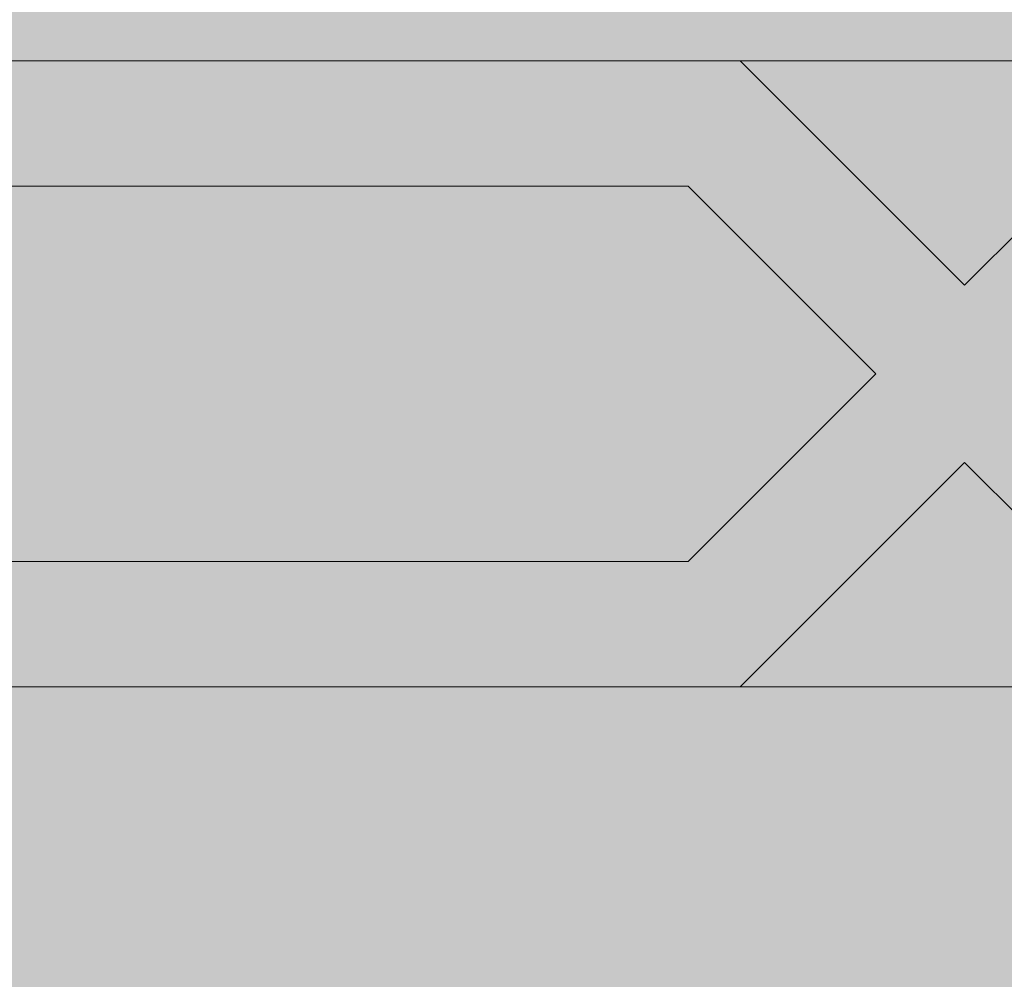
# Model space of a CAD drawing. Units: inches. Extents: x 844 to 2234, y 346 to 1084.
# Tile 81 of 93: x 2001.933 to 2003.94, y 710.971 to 712.926. Entities that reach past the tile are written whole.
import ezdxf

# ---------------------------------------------------------------- set-up
doc = ezdxf.new("R2010")
doc.units = ezdxf.units.IN
doc.header["$MEASUREMENT"] = 0
for name, color, linetype, lineweight in [('A-ANNO-DIMS', 2, 'Continuous', 18), ('furniture', 8, 'Continuous', 18), ('RA-AP-01$0$INT', 35, 'Continuous', 5)]:
    doc.layers.add(name, color=color, linetype=linetype, lineweight=lineweight)
doc.layers.add('RA-AP-01$0$FURN', color=3, linetype='Continuous')
doc.styles.get("Standard").update_dxf_attribs({"font": 'arial.ttf'})
doc.dimstyles.get("Standard").update_dxf_attribs({"dimtxt": 6, "dimasz": 3, "dimexe": 0.18, "dimexo": 0.0625, "dimgap": 0.09, "dimtad": 0, "dimtih": 1, "dimtoh": 1, "dimdec": 1, "dimzin": 0, "dimdsep": 46, "dimlunit": 3, "dimtxsty": 'Standard', "dimblk": 'ARCHTICK', "dimcen": 0.09, "dimadec": 0, "dimazin": 0, "dimtfac": 1, "dimtdec": 1, "dimtofl": 0, "dimtmove": 0, "dimatfit": 3, "dimfxl": 1, "dimtolj": 1, "dimtzin": 0, "dimarcsym": 0})

# ---------------------------------------------------------------- blocks, each defined once
blk = doc.blocks.new('A$C18D01794')
at = {"layer": 'RA-AP-01$0$INT'}
h = blk.add_hatch(color=256, dxfattribs=at)
h.paths.add_polyline_path([(4.355206456958071, -6.156712009588037), (4.355206456958071, -8.056712009588038), (5.455206456958072, -8.056712009588038), (5.455206456958072, -6.156712009588037)])
h.paths.add_polyline_path([(4.405206456958072, -8.006712009588039), (4.405206456958072, -6.206712009588038), (5.405206456958072, -6.206712009588038), (5.405206456958072, -8.006712009588039)], flags=16)
h = blk.add_hatch(color=256, dxfattribs=at)
h.paths.add_polyline_path([(4.505206456958071, -7.585498806127123), (4.46934859260189, -7.549640941759413), (4.505206456958071, -7.513783077414768), (4.505206456958071, -7.381963272220687), (4.469348592616735, -7.346105407867824), (4.505206456958071, -7.310247543514964), (4.505206456958071, -7.178427738324996), (4.469348592586679, -7.142569873965138), (4.505206456952245, -7.106712009588038), (4.476922185709333, -7.106712009588038), (4.455206456960671, -7.128427738343681), (4.433490728198047, -7.106712009588038), (4.405206456946033, -7.106712009588036), (4.441064321339216, -7.142569873969684), (4.40520645695807, -7.178427738362358), (4.405206456958072, -7.310247543472698), (4.441064321364728, -7.346105407867826), (4.40520645695807, -7.381963272262947), (4.40520645695807, -7.513783077378263), (4.441064321354429, -7.549640941786153), (4.405206456958072, -7.585498806170974), (4.405206456958072, -7.717318611286652), (4.441064321333084, -7.753176475673194), (4.405206456958072, -7.789034340036673), (4.405206456958072, -8.006712009588039), (4.644348592588106, -8.006712009588039), (4.680206456964639, -7.970854145211967), (4.716064321341165, -8.006712009588039), (4.869348592586113, -8.006712009588039), (4.905206456964143, -7.970854145210465), (4.941064321342174, -8.006712009588039), (5.094348592587118, -8.006712009588037), (5.130206456963649, -7.970854145211967), (5.166064321340178, -8.006712009588039), (5.405206456958072, -8.006712009588039), (5.405206456958072, -7.789034340024526), (5.369348592595202, -7.753176475673196), (5.40520645695807, -7.717318611298797), (5.40520645695807, -7.585498806158829), (5.369348592573859, -7.549640941786151), (5.40520645695807, -7.51378307739041), (5.40520645695807, -7.381963272250803), (5.36934859256356, -7.346105407867824), (5.405206456958072, -7.310247543484846), (5.405206456958072, -7.178427738350217), (5.369348592589068, -7.142569873969682), (5.405206456982249, -7.106712009588038), (5.376922185730244, -7.106712009588038), (5.355206456967613, -7.128427738343679), (5.333490728218955, -7.10671200958804), (5.305206456976043, -7.106712009588042), (5.341064321341609, -7.142569873965136), (5.305206456958072, -7.178427738337141), (5.305206456958072, -7.310247543502816), (5.34106432131155, -7.346105407867824), (5.305206456958072, -7.381963272232832), (5.30520645695807, -7.513783077402624), (5.341064321326395, -7.549640941759413), (5.305206456958072, -7.585498806139263), (5.305206456958072, -7.717318611299605), (5.341064321347738, -7.753176475677737), (5.305206456958072, -7.78903434007894), (5.30520645695807, -7.906712009588039), (5.166064321336834, -7.906712009588039), (5.130206456963647, -7.942569873961684), (5.094348592590464, -7.906712009588039), (4.941064321338827, -7.906712009588041), (4.905206456964145, -7.942569873963183), (4.869348592589459, -7.906712009588039), (4.716064321337822, -7.906712009588041), (4.680206456964641, -7.942569873961684), (4.644348592591453, -7.906712009588039), (4.505206456958071, -7.906712009588039), (4.505206456958071, -7.789034340066795), (4.469348592580545, -7.753176475677738), (4.505206456958071, -7.717318611311748)])
h.paths.add_polyline_path([(4.485206456974132, -7.709034340046354), (4.45520645695909, -7.739034340051736), (4.425206456974128, -7.709034340057131), (4.425206456993394, -7.593783077384998), (4.45520645699153, -7.563783077396511), (4.485206456993396, -7.593783077408017)], flags=16)
h.paths.add_polyline_path([(4.455206456954537, -7.767318611299197), (4.485206456958242, -7.797318611312542), (4.48520645695951, -7.912569873958716), (4.45520645695415, -7.942569873954422), (4.425206456957888, -7.912569873967813), (4.425206456957888, -7.797318611286197)], flags=16)
h.paths.add_polyline_path([(4.455206456964794, -7.535498806149051), (4.42520645696469, -7.5054988061393), (4.425206456983954, -7.390247543486406), (4.455206456990734, -7.360247543489279), (4.485206456983953, -7.39024754349214), (4.485206456964687, -7.505498806158811)], flags=16)
h.paths.add_polyline_path([(4.499348592588947, -7.926712009585049), (4.636064321340932, -7.926712009585049), (4.666064321342317, -7.956712009586821), (4.636064321343707, -7.986712009585048), (4.499348592575121, -7.986712009585048), (4.469348592591685, -7.956712009591957)], flags=16)
h.paths.add_polyline_path([(4.425206456957888, -7.940854145195974), (4.471064321332215, -7.986712009585049), (4.425206456957888, -7.986712009585049)], flags=16)
h.paths.add_polyline_path([(4.455206456990734, -7.331963272246367), (4.425206456989053, -7.301963272254337), (4.425206456969784, -7.186712009596224), (4.455206456965226, -7.156712009591144), (4.485206456969787, -7.186712009586051), (4.485206456989053, -7.301963272238404)], flags=16)
h.paths.add_polyline_path([(4.72434859258714, -7.926712009586255), (4.861064321340141, -7.926712009586248), (4.891064321340324, -7.956712009586823), (4.861064321340513, -7.986712009586252), (4.724348592586768, -7.986712009586252), (4.694348592586956, -7.956712009586821)], flags=16)
h.paths.add_polyline_path([(4.919348592587961, -7.956712009586821), (4.949348592588145, -7.92671200958625), (5.08606432134115, -7.926712009586253), (5.116064321341327, -7.956712009586823), (5.086064321341519, -7.986712009586252), (4.949348592587774, -7.986712009586252)], flags=16)
h.paths.add_polyline_path([(5.144348592585967, -7.956712009586823), (5.174348592587358, -7.926712009585049), (5.311064321339338, -7.926712009585049), (5.3410643213366, -7.956712009591957), (5.311064321353163, -7.986712009585048), (5.174348592584576, -7.986712009585048)], flags=16)
h.paths.add_polyline_path([(5.32520645693489, -7.593783077408021), (5.355206456936755, -7.563783077396511), (5.385206456934894, -7.593783077384998), (5.38520645695416, -7.709034340057128), (5.355206456969194, -7.739034340051736), (5.325206456954153, -7.709034340046352)], flags=16)
h.paths.add_polyline_path([(5.325206456970042, -7.797318611312542), (5.355206456973747, -7.767318611299197), (5.385206456970398, -7.7973186112862), (5.385206456970398, -7.912569873967816), (5.355206456974136, -7.942569873954422), (5.325206456968778, -7.912569873958716)], flags=16)
h.paths.add_polyline_path([(5.325206456963599, -7.505498806158811), (5.325206456944333, -7.39024754349214), (5.355206456937552, -7.360247543489279), (5.385206456944332, -7.39024754348641), (5.385206456963596, -7.505498806139303), (5.355206456963492, -7.53549880614905)], flags=16)
h.paths.add_polyline_path([(5.32520645693923, -7.301963272238403), (5.3252064569585, -7.186712009586051), (5.355206456963062, -7.156712009591142), (5.3852064569585, -7.186712009596224), (5.385206456939234, -7.301963272254338), (5.355206456937552, -7.331963272246369)], flags=16)
h.paths.add_polyline_path([(5.339348592596071, -7.986712009585048), (5.385206456970398, -7.940854145195972), (5.385206456970396, -7.986712009585048)], flags=16)
h = blk.add_hatch(color=256, dxfattribs=at)
h.paths.add_polyline_path([(4.469348592586677, -7.142569873965136), (4.505206456958073, -7.178427738324996), (4.505206456958071, -7.106712009582215)])
h.paths.add_polyline_path([(4.455206456960671, -7.128427738343681), (4.476922185709333, -7.106712009588038), (4.433490728198045, -7.106712009588038)])
h.paths.add_polyline_path([(4.405206456958073, -7.178427738362358), (4.441064321339218, -7.142569873969684), (4.40520645695807, -7.106712009600073)])
h.paths.add_polyline_path([(4.425206456989053, -7.301963272254335), (4.455206456990736, -7.331963272246371), (4.485206456989055, -7.301963272238399), (4.48520645696979, -7.186712009586054), (4.455206456965227, -7.15671200959114), (4.425206456969784, -7.186712009596224)])
h.paths.add_polyline_path([(4.505206456958073, -7.381963272220689), (4.505206456958071, -7.310247543514961), (4.469348592616738, -7.346105407867826)])
h.paths.add_polyline_path([(4.425206456964688, -7.5054988061393), (4.455206456964794, -7.535498806149051), (4.485206456964689, -7.505498806158811), (4.485206456983951, -7.390247543492138), (4.455206456990736, -7.360247543489277), (4.425206456983956, -7.39024754348641)])
h.paths.add_polyline_path([(4.425206456974126, -7.709034340057128), (4.455206456959092, -7.739034340051736), (4.485206456974132, -7.709034340046356), (4.485206456993396, -7.593783077408017), (4.45520645699153, -7.563783077396511), (4.425206456993394, -7.593783077384999)])
h.paths.add_polyline_path([(4.46934859260189, -7.549640941759415), (4.505206456958071, -7.585498806127123), (4.505206456958073, -7.513783077414766)])
h.paths.add_polyline_path([(4.405206456958073, -7.585498806170972), (4.441064321354427, -7.549640941786151), (4.405206456958072, -7.513783077378263)])
h.paths.add_polyline_path([(4.405206456958072, -7.789034340036673), (4.441064321333084, -7.753176475673194), (4.405206456958072, -7.71731861128665)])
h.paths.add_polyline_path([(4.469348592580547, -7.75317647567774), (4.505206456958071, -7.789034340066795), (4.505206456958071, -7.717318611311744)])
h.paths.add_polyline_path([(4.425206456957888, -7.912569873967814), (4.45520645695415, -7.942569873954422), (4.485206456959507, -7.912569873958718), (4.48520645695824, -7.797318611312542), (4.455206456954537, -7.767318611299197), (4.425206456957888, -7.797318611286202)])
h.paths.add_polyline_path([(4.425206456957888, -7.986712009585049), (4.471064321332215, -7.986712009585049), (4.425206456957888, -7.940854145195972)])
h.paths.add_polyline_path([(4.499348592575121, -7.986712009585048), (4.636064321343707, -7.986712009585049), (4.666064321342317, -7.956712009586823), (4.636064321340932, -7.926712009585049), (4.499348592588945, -7.926712009585049), (4.469348592591685, -7.95671200959196)])
h.paths.add_polyline_path([(4.680206456964641, -7.942569873961684), (4.716064321337824, -7.906712009588039), (4.644348592591454, -7.906712009588039)])
h.paths.add_polyline_path([(4.644348592588108, -8.006712009588039), (4.716064321341167, -8.006712009588039), (4.680206456964637, -7.970854145211964)])
h.paths.add_polyline_path([(4.724348592586768, -7.98671200958625), (4.861064321340514, -7.986712009586252), (4.891064321340324, -7.956712009586819), (4.861064321340141, -7.92671200958625), (4.724348592587134, -7.926712009586255), (4.694348592586957, -7.956712009586821)])
h.paths.add_polyline_path([(4.905206456964143, -7.942569873963183), (4.941064321338827, -7.906712009588039), (4.869348592589457, -7.906712009588037)])
h.paths.add_polyline_path([(4.869348592586113, -8.006712009588039), (4.941064321342172, -8.006712009588037), (4.905206456964145, -7.970854145210463)])
h.paths.add_polyline_path([(4.949348592587774, -7.986712009586252), (5.086064321341521, -7.986712009586252), (5.116064321341329, -7.956712009586823), (5.08606432134115, -7.926712009586253), (4.949348592588145, -7.92671200958625), (4.919348592587961, -7.956712009586819)])
h.paths.add_polyline_path([(5.130206456963645, -7.942569873961684), (5.166064321336834, -7.906712009588039), (5.094348592590464, -7.906712009588039)])
h.paths.add_polyline_path([(5.094348592587119, -8.006712009588039), (5.166064321340178, -8.006712009588039), (5.130206456963651, -7.970854145211967)])
h.paths.add_polyline_path([(5.174348592584578, -7.986712009585048), (5.311064321353163, -7.986712009585048), (5.341064321336602, -7.956712009591958), (5.31106432133934, -7.926712009585049), (5.174348592587352, -7.926712009585049), (5.144348592585969, -7.956712009586823)])
h.paths.add_polyline_path([(5.325206456968778, -7.912569873958718), (5.355206456974136, -7.942569873954422), (5.385206456970396, -7.912569873967814), (5.385206456970396, -7.797318611286199), (5.355206456973747, -7.767318611299197), (5.325206456970044, -7.797318611312544)])
h.paths.add_polyline_path([(5.339348592596073, -7.986712009585048), (5.385206456970396, -7.986712009585049), (5.385206456970398, -7.94085414519597)])
h.paths.add_polyline_path([(5.325206456954155, -7.709034340046354), (5.355206456969194, -7.739034340051734), (5.38520645695416, -7.709034340057128), (5.385206456934896, -7.593783077384999), (5.355206456936758, -7.563783077396513), (5.325206456934888, -7.593783077408019)])
h.paths.add_polyline_path([(5.305206456958072, -7.789034340078938), (5.341064321347739, -7.753176475677738), (5.305206456958072, -7.717318611299605)])
h.paths.add_polyline_path([(5.369348592595204, -7.753176475673194), (5.40520645695807, -7.789034340024526), (5.405206456958072, -7.717318611298798)])
h.paths.add_polyline_path([(5.405206456958072, -7.585498806158831), (5.405206456958072, -7.513783077390407), (5.369348592573857, -7.549640941786151)])
h.paths.add_polyline_path([(5.305206456958072, -7.585498806139266), (5.341064321326393, -7.549640941759413), (5.305206456958072, -7.513783077402626)])
h.paths.add_polyline_path([(5.325206456963599, -7.50549880615881), (5.355206456963494, -7.535498806149055), (5.385206456963598, -7.505498806139302), (5.385206456944334, -7.390247543486411), (5.355206456937552, -7.360247543489279), (5.325206456944333, -7.39024754349214)])
h.paths.add_polyline_path([(5.305206456958072, -7.38196327223283), (5.341064321311551, -7.346105407867824), (5.305206456958072, -7.31024754350282)])
h.paths.add_polyline_path([(5.325206456939231, -7.301963272238404), (5.355206456937552, -7.331963272246369), (5.385206456939235, -7.301963272254335), (5.385206456958502, -7.186712009596224), (5.355206456963061, -7.156712009591142), (5.3252064569585, -7.186712009586051)])
h.paths.add_polyline_path([(5.404581768715993, -7.381338584008926, -0.001217816984214), (5.405206456958072, -7.381112009582329), (5.405206456958072, -7.310247543484846), (5.369348592563558, -7.346105407867826)])
h.paths.add_polyline_path([(5.36934859258907, -7.142569873969684), (5.40520645695807, -7.178427738350215), (5.405206456958072, -7.106712009612218)])
h.paths.add_polyline_path([(5.355206456967613, -7.128427738343683), (5.376922185730239, -7.106712009588038), (5.333490728218953, -7.10671200958804)])
h.paths.add_polyline_path([(5.30520645695807, -7.178427738337139), (5.341064321341609, -7.142569873965134), (5.305206456958074, -7.10671200957007)])
blk.add_hatch(color=256, dxfattribs=at).paths.add_polyline_path([(4.505206456958071, -7.906712009588039), (5.305206456958072, -7.906712009588039), (5.305206456958072, -7.106712009588038), (5.255206456951893, -7.106712009588036), (5.25520645694868, -7.856712009570104), (4.555206456959269, -7.856712009588616), (4.555206456956052, -7.106712009588038), (4.505206456958073, -7.106712009588038)])
for p, q in [((5.267206456961765, -7.906712009586254), (4.543206456966523, -7.906712009586254)), ((5.2672064569642, -7.906712009586255), (4.54320645696085, -7.906712009586255)), ((4.869348592587674, -7.906712009586254), (4.905206456964143, -7.942569873963183)), ((4.941064321340612, -7.906712009586254), (4.905206456964143, -7.942569873963183)), ((4.949348592588145, -7.92671200958625), (4.919348592587962, -7.956712009586821)), ((4.949348592588145, -7.92671200958625), (5.08606432134115, -7.926712009586253)), ((4.949348592587774, -7.986712009586252), (4.919348592587962, -7.956712009586821)), ((4.8693485925879, -8.006712009586252), (4.905206456964143, -7.970854145210465)), ((4.941064321340387, -8.006712009586252), (4.905206456964143, -7.970854145210465)), ((4.949348592587774, -7.986712009586252), (5.086064321341518, -7.986712009586252))]:
    blk.add_line(p, q, dxfattribs=at)
for points in [[(5.405206456958072, -8.006712009588039), (4.405206456958072, -8.006712009588039), (4.405206456958072, -7.106712009588038)], [(5.305206456958072, -7.106712009588038), (5.305206456958072, -7.906712009588039), (4.505206456958071, -7.906712009588039), (4.505206456958071, -7.106712009588038)]]:
    blk.add_lwpolyline(points, dxfattribs=at)
blk = doc.blocks.new('A$C5D2F253E')
at = {"layer": 'RA-AP-01$0$FURN', "xscale": -0.7999999999883585, "yscale": 0.7999999999883585, "zscale": 0.8, "rotation": 90}
blk.add_blockref('A$C18D01794', (-5.687757199772477, 4.75791982714071), dxfattribs=at)
blk = doc.blocks.new('_ArchTick')
at = {"color": 0, "linetype": 'ByBlock', "const_width": 0.15}
blk.add_lwpolyline([(-0.5, -0.5), (0.5, 0.5)], dxfattribs=at)
blk = doc.blocks.new('*D121')
at = {"layer": 'A-ANNO-DIMS', "color": 0, "lineweight": -2, "transparency": 16777216}
for p, q in [((2030.271987351997, 734.262611118704), (2040.245275089302, 734.262611118704)), ((2040.065275089302, 734.262611118704), (2040.065275089302, 704.6043509484256)), ((2040.065275089302, 668.557359536674), (2040.065275089302, 698.2156197069523)), ((2030.271987351997, 668.557359536674), (2040.245275089302, 668.557359536674))]:
    blk.add_line(p, q, dxfattribs=at)
at = {"layer": 'Defpoints', "color": 0, "transparency": 16777216}
for p in [(2030.209487351997, 734.262611118704), (2040.065275089302, 734.262611118704), (2030.209487351997, 668.557359536674)]:
    blk.add_point(p, dxfattribs=at)
at = {"layer": 'A-ANNO-DIMS', "color": 0, "lineweight": -2, "transparency": 16777216, "xscale": 3, "yscale": 3, "zscale": 3}
for p, rotation in [((2040.065275089302, 734.262611118704), 90), ((2040.065275089302, 668.557359536674), 270)]:
    blk.add_blockref('_ArchTick', p, dxfattribs=dict(at, rotation=rotation))
at = {"layer": 'A-ANNO-DIMS', "color": 0, "transparency": 16777216, "insert": (2040.065275089302, 701.4099853276883), "char_height": 6, "attachment_point": 5}
blk.add_mtext('\\A1;LOUNGE SET 5\'-5 1/2" TYP.', dxfattribs=at)

msp = doc.modelspace()

# ---------------------------------------------------------------- block references
at = {"layer": 'furniture', "xscale": -15.94108302203742, "yscale": 15.94108302203742, "zscale": 15.94108302203742, "rotation": 270}
msp.add_blockref('A$C5D2F253E', (1990.567271852805, 701.4028671565849), dxfattribs=at)

# ---------------------------------------------------------------- dimensions: what is measured, and where the dimension line sits
at = {"layer": 'A-ANNO-DIMS'}
dim = msp.add_linear_dim(base=(2040.065275089302, 734.262611118704), p1=(2030.209487351996, 668.5573595366737), p2=(2030.209487351996, 734.2626111187037), angle=90, text='LOUNGE SET <> TYP.', dimstyle='Standard', override={"dimdec": 1, "dimlfac": 1, "dimrnd": 0, "dimzin": 1, "dimdsep": 46, "dimlunit": 4, "dimfrac": 2}, dxfattribs=at)
dim.commit()
dim.dimension.update_dxf_attribs({"geometry": '*D121', "text_midpoint": (2040.065275089302, 701.4099853276883)})

doc.saveas('drawing.dxf')
